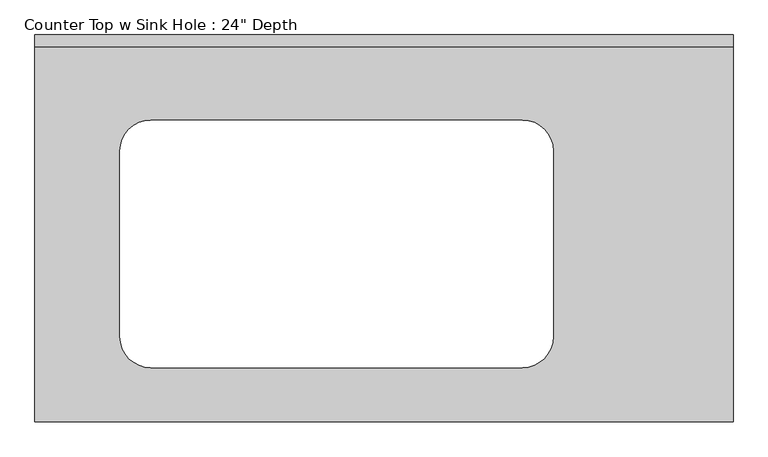
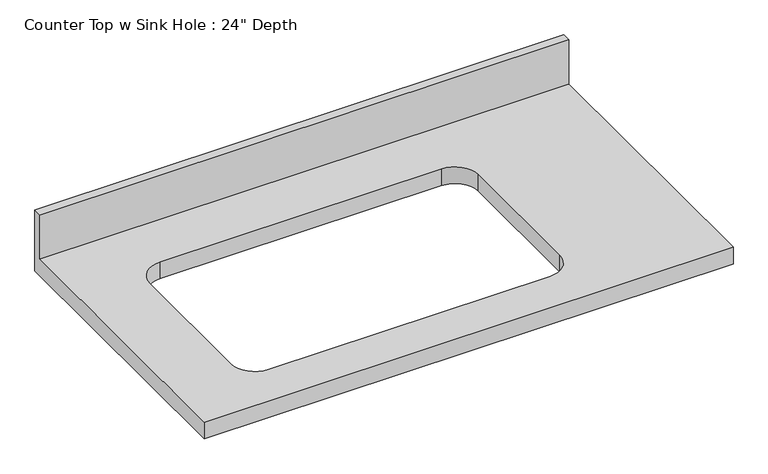
"""IFC4 building model written with IfcOpenShell, lengths in millimetres: furniture geometry."""

from ifc_helpers import new_model, si_unit, frame, origin, place, context, project, spatial, polyline, circle_curve, source, transform, mapped, element, save
from ifc_brep_helpers import plane_surface, revolved_surface, advanced_brep


def furniture_ce4e80af(model_context):
    return source(origin(), model_context, "Body", "AdvancedBrep", [
        advanced_brep(
        [(-1200.4622951, -635.0, 914.4), (-54.4174038, -635.0, 914.4), (-54.4174038, -19.05, 914.4), (-1200.4622951, -19.05, 914.4), (-1010.093936, -139.7, 914.4), (-400.493936, -139.7, 914.4), (-349.693936, -190.5, 914.4), (-349.693936, -495.3, 914.4), (-400.493936, -546.1, 914.4), (-1010.093936, -546.1, 914.4), (-1060.893936, -495.3, 914.4), (-1060.893936, -190.5, 914.4), (-54.4174038, 0.0, 876.3), (-54.4174038, -635.0, 876.3), (-1200.4622951, -635.0, 876.3), (-1200.4622951, 0.0, 876.3), (-400.493936, -139.7, 876.3), (-1010.093936, -139.7, 876.3), (-1060.893936, -190.5, 876.3), (-1060.893936, -495.3, 876.3), (-1010.093936, -546.1, 876.3), (-400.493936, -546.1, 876.3), (-349.693936, -495.3, 876.3), (-349.693936, -190.5, 876.3), (-1200.4622951, 0.0, 1016.0), (-54.4174038, 0.0, 1016.0), (-1200.4622951, -19.05, 1016.0), (-54.4174038, -19.05, 1016.0)],
        [
            (0, 1),
            (1, 2),
            (2, 3),
            (3, 0),
            (4, 5),
            (5, 6, circle_curve(frame((-400.493936, -190.5, 914.4), z_axis=(0.0, 0.0, -1.0), x_axis=(1.0, 0.0, 0.0)), 50.8)),
            (6, 7),
            (7, 8, circle_curve(frame((-400.493936, -495.3, 914.4), z_axis=(0.0, 0.0, -1.0), x_axis=(1.0, 0.0, 0.0)), 50.8)),
            (8, 9),
            (9, 10, circle_curve(frame((-1010.093936, -495.3, 914.4), z_axis=(0.0, 0.0, -1.0), x_axis=(1.0, 0.0, 0.0)), 50.8)),
            (10, 11),
            (11, 4, circle_curve(frame((-1010.093936, -190.5, 914.4), z_axis=(0.0, 0.0, -1.0), x_axis=(1.0, 0.0, 0.0)), 50.8)),
            (12, 13),
            (13, 14),
            (14, 15),
            (15, 12),
            (16, 17),
            (17, 18, circle_curve(frame((-1010.093936, -190.5, 876.3), z_axis=(0.0, 0.0, 1.0), x_axis=(1.0, 0.0, 0.0)), 50.8)),
            (18, 19),
            (19, 20, circle_curve(frame((-1010.093936, -495.3, 876.3), z_axis=(0.0, 0.0, 1.0), x_axis=(1.0, 0.0, 0.0)), 50.8)),
            (20, 21),
            (21, 22, circle_curve(frame((-400.493936, -495.3, 876.3), z_axis=(0.0, 0.0, 1.0), x_axis=(1.0, 0.0, 0.0)), 50.8)),
            (22, 23),
            (23, 16, circle_curve(frame((-400.493936, -190.5, 876.3), z_axis=(0.0, 0.0, 1.0), x_axis=(1.0, 0.0, 0.0)), 50.8)),
            (15, 24),
            (24, 25),
            (25, 12),
            (14, 0),
            (3, 26),
            (26, 24),
            (13, 1),
            (25, 27),
            (27, 2),
            (26, 27),
            (4, 17),
            (16, 5),
            (11, 18),
            (10, 19),
            (9, 20),
            (8, 21),
            (7, 22),
            (6, 23),
        ],
        [
            plane_surface(frame((-1200.4622951, 0.0, 914.4), z_axis=(0.0, 0.0, 1.0), x_axis=(-1.0, 0.0, 0.0))),
            plane_surface(frame((-1200.4622951, 0.0, 876.3), z_axis=(0.0, 0.0, -1.0), x_axis=(1.0, 0.0, 0.0))),
            plane_surface(frame((-54.4174038, 0.0, 914.4), z_axis=(0.0, 1.0, 0.0), x_axis=(0.0, 0.0, -1.0))),
            plane_surface(frame((-1200.4622951, 0.0, 914.4), z_axis=(-1.0, 0.0, 0.0), x_axis=(0.0, 0.0, -1.0))),
            plane_surface(frame((-1200.4622951, -635.0, 914.4), z_axis=(0.0, -1.0, 0.0), x_axis=(0.0, 0.0, -1.0))),
            plane_surface(frame((-54.4174038, -635.0, 914.4), z_axis=(1.0, 0.0, 0.0), x_axis=(0.0, 0.0, -1.0))),
            plane_surface(frame((-1200.4622951, 0.0, 1016.0), z_axis=(0.0, 0.0, 1.0), x_axis=(0.0, -1.0, 0.0))),
            plane_surface(frame((-1200.4622951, -19.05, 1016.0), z_axis=(0.0, -1.0, 0.0), x_axis=(0.0, 0.0, -1.0))),
            plane_surface(frame((-400.493936, -139.7, 914.4), z_axis=(0.0, -1.0, 0.0), x_axis=(0.0, 0.0, -1.0))),
            revolved_surface(polyline([(-959.293936, -190.5, 914.4), (-959.293936, -190.5, 876.3)]), (-1010.093936, -190.5, 876.3), (0.0, 0.0, 1.0)),
            plane_surface(frame((-1060.893936, -190.5, 914.4), z_axis=(1.0, 0.0, 0.0), x_axis=(0.0, 0.0, -1.0))),
            revolved_surface(polyline([(-959.293936, -495.3, 914.4), (-959.293936, -495.3, 876.3)]), (-1010.093936, -495.3, 876.3), (0.0, 0.0, 1.0)),
            plane_surface(frame((-1010.093936, -546.1, 914.4), z_axis=(0.0, 1.0, 0.0), x_axis=(0.0, 0.0, -1.0))),
            revolved_surface(polyline([(-349.693936, -495.3, 914.4), (-349.693936, -495.3, 876.3)]), (-400.493936, -495.3, 876.3), (0.0, 0.0, 1.0)),
            plane_surface(frame((-349.693936, -495.3, 914.4), z_axis=(-1.0, 0.0, 0.0), x_axis=(0.0, 0.0, -1.0))),
            revolved_surface(polyline([(-349.693936, -190.5, 914.4), (-349.693936, -190.5, 876.3)]), (-400.493936, -190.5, 876.3), (0.0, 0.0, 1.0)),
        ],
        [
            (0, [[1, 2, 3, 4], [5, 6, 7, 8, 9, 10, 11, 12]]),
            (1, [[13, 14, 15, 16], [17, 18, 19, 20, 21, 22, 23, 24]]),
            (2, [[-16, 25, 26, 27]]),
            (3, [[-15, 28, -4, 29, 30, -25]]),
            (4, [[-1, -28, -14, 31]]),
            (5, [[-13, -27, 32, 33, -2, -31]]),
            (6, [[-30, 34, -32, -26]]),
            (7, [[-34, -29, -3, -33]]),
            (8, [[35, -17, 36, -5]]),
            (9, [[-35, -12, 37, -18]]),
            (10, [[-37, -11, 38, -19]]),
            (11, [[-38, -10, 39, -20]]),
            (12, [[-39, -9, 40, -21]]),
            (13, [[-40, -8, 41, -22]]),
            (14, [[-41, -7, 42, -23]]),
            (15, [[-36, -24, -42, -6]]),
        ],
    ),
    ])


if __name__ == "__main__":
    model = new_model("IFC4")
    model_context = context("Model", 3, world=origin())
    ifc_project = project(units=[si_unit("LENGTHUNIT", "METRE", prefix="MILLI")], contexts=[model_context])
    site = spatial("IfcSite", under=ifc_project)
    building = spatial("IfcBuilding", under=site)
    placement = place(None, origin())
    furniture_shape = furniture_ce4e80af(model_context)
    element("IfcFurniture", 1, ObjectType="Counter Top w Sink Hole : 24\" Depth", at=placement, inside=building, context=model_context, shape_type="MappedRepresentation", body=[
        mapped(furniture_shape, transform((0.0, 0.0, 0.0), x_axis=(1.0, 0.0, 0.0), y_axis=(0.0, 1.0, 0.0), z_axis=(0.0, 0.0, 1.0))),
    ])
    save(model, "model.ifc")

# Revit data of these elements
# Type "Counter Top w Sink Hole : 24\" Depth"
#   Assembly Code = "C1030400"
#   Counter Thickness = 0' - 1 1/2"
#   Depth = 2' - 1"
#   Height = 3' - 0"
#   Length [instance default] = 8' - 0"
#   Sink Location [instance default] = 2' - 0"
#   Sink Location To Wall [instance default] = 0' - 6"
#   Sink Opening Depth [instance default] = 1' - 3"
#   Sink Opening Width [instance default] = 2' - 3"
#   Counter Top Material = none
#   Default Elevation = 0
# Element 1 (IfcFurniture, "Counter Top w Sink Hole : 24\" Depth")
#   Length = 3' - 9.11988"
#   Sink Location = 1' - 7.49482"
#   Materials on its faces: "Counter Top"
# Materials
#   "Counter Top": class "Wood", colour RGB 226 177 128, transparency 0
